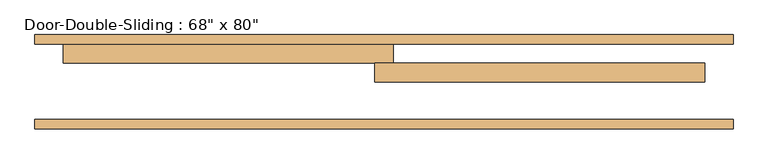
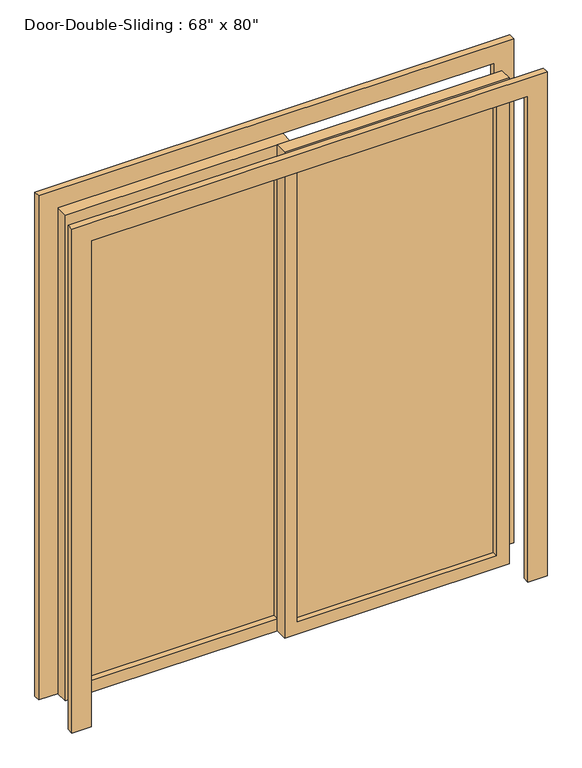
"""IFC4 building model written with IfcOpenShell, lengths in millimetres: door geometry."""

from ifc_helpers import new_model, si_unit, frame, origin, place, context, project, spatial, polyline, outline, extrude, source, transform, mapped, element, save


def door_076b30e0(model_context):
    return source(origin(), model_context, "Body", "SweptSolid", [
        extrude(outline(polyline([(0.0, -939.8), (0.0, -863.6), (2032.0, -863.6), (2032.0, 863.6), (0.0, 863.6), (0.0, 939.8), (2108.2, 939.8), (2108.2, -939.8), (0.0, -939.8)])), frame((0.0, 0.0, 0.0), z_axis=(0.0, 1.0, 0.0), x_axis=(0.0, 0.0, 1.0)), (0.0, 0.0, 1.0), 25.4),
        extrude(outline(polyline([(0.0, 939.8), (2108.2, 939.8), (2108.2, -939.8), (0.0, -939.8), (0.0, -863.6), (2032.0, -863.6), (2032.0, 863.6), (0.0, 863.6), (0.0, 939.8)])), frame((0.0, 228.6, 0.0), z_axis=(0.0, 1.0, 0.0), x_axis=(0.0, 0.0, 1.0)), (0.0, 0.0, 1.0), 25.4),
        extrude(outline(polyline([(2032.0, -25.4), (0.0, -25.4), (0.0, 863.6), (2032.0, 863.6), (2032.0, -25.4)]), holes=[polyline([(1981.2, 25.4), (1981.2, 812.8), (50.8, 812.8), (50.8, 25.4), (1981.2, 25.4)])]), frame((0.0, 127.0, 0.0), z_axis=(0.0, 1.0, 0.0), x_axis=(0.0, 0.0, 1.0)), (0.0, 0.0, 1.0), 50.8),
        extrude(outline(polyline([(2032.0, 25.4), (2032.0, -863.6), (0.0, -863.6), (0.0, 25.4), (2032.0, 25.4)]), holes=[polyline([(1981.2, -25.4), (50.8, -25.4), (50.8, -812.8), (1981.2, -812.8), (1981.2, -25.4)])]), frame((0.0, 177.8, 0.0), z_axis=(0.0, 1.0, 0.0), x_axis=(0.0, 0.0, 1.0)), (0.0, 0.0, 1.0), 50.8),
        extrude(outline(polyline([(25.4, 155.575), (812.8, 155.575), (812.8, 149.225), (25.4, 149.225), (25.4, 155.575)])), frame((0.0, 0.0, 50.8), z_axis=(0.0, 0.0, 1.0), x_axis=(1.0, 0.0, 0.0)), (0.0, 0.0, 1.0), 1930.4),
        extrude(outline(polyline([(-25.4, 200.025), (-812.8, 200.025), (-812.8, 206.375), (-25.4, 206.375), (-25.4, 200.025)])), frame((0.0, 0.0, 50.8), z_axis=(0.0, 0.0, 1.0), x_axis=(1.0, 0.0, 0.0)), (0.0, 0.0, 1.0), 1930.4),
    ])


if __name__ == "__main__":
    model = new_model("IFC4")
    model_context = context("Model", 3, world=origin())
    ifc_project = project(units=[si_unit("LENGTHUNIT", "METRE", prefix="MILLI")], contexts=[model_context])
    site = spatial("IfcSite", under=ifc_project)
    building = spatial("IfcBuilding", under=site)
    placement = place(None, origin())
    door_shape = door_076b30e0(model_context)
    element("IfcDoor", 1, ObjectType="Door-Double-Sliding : 68\" x 80\"", at=placement, inside=building, context=model_context, shape_type="MappedRepresentation", body=[
        mapped(door_shape, transform((0.0, 0.0, 0.0), x_axis=(1.0, 0.0, 0.0), y_axis=(0.0, 1.0, 0.0), z_axis=(0.0, 0.0, 1.0))),
    ])
    save(model, "model.ifc")

# Revit data of these elements
# Type "Door-Double-Sliding : 68\" x 80\""
#   Type Mark = "10"
#   Construction Type Id = "opn-d45"
#   Assembly Code = "C1020"
#   Analytic Construction = "Wood frame, double glass door "
#   Thickness = 0' - 2"
#   Thermal Resistance (R) = 1.8150 (h·ft²·°F)/BTU
#   Heat Transfer Coefficient (U) = 0.5510 BTU/(h·ft²·°F)
#   Height = 6' - 8"
#   Rail Width = 0' - 2"
#   Stiles = 0' - 2"
#   Trim Projection Ext = 0' - 1"
#   Trim Projection Int = 0' - 1"
#   Trim Width = 0' - 3"
#   Width = 5' - 8"
#   Define Thermal Properties by = 1
#   Glazing = Glass
#   Panel Material = Wood - Birch - Solid Stained Light Low Gloss
#   Trim Material = Paint - Sienna
#   Visual Light Transmittance = 0
#   Solar Heat Gain Coefficient = 0
#   Function = (empty or 0)
#   Wall Closure = (empty or 0)
# Element 1 (IfcDoor, "Door-Double-Sliding : 68\" x 80\"")
#   Materials on its faces: "Paint - Sienna", "Wood - Birch - Solid Stained Light Low Gloss", "Glass"
# Materials
#   "Glass": class "Glass", colour RGB 0 128 192, transparency 0.75, Description = "Soda Lime Glass", Cost = 0
#   "Wood - Birch - Solid Stained Light Low Gloss": class "Wood", colour RGB 210 159 95, transparency 0, Cost = 0
#   "Paint - Sienna": colour RGB 118 70 51, transparency 0, Cost = 0
